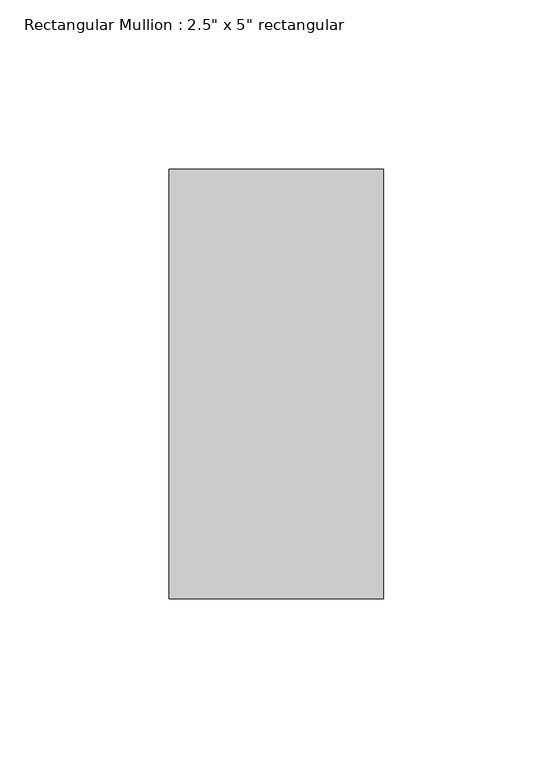
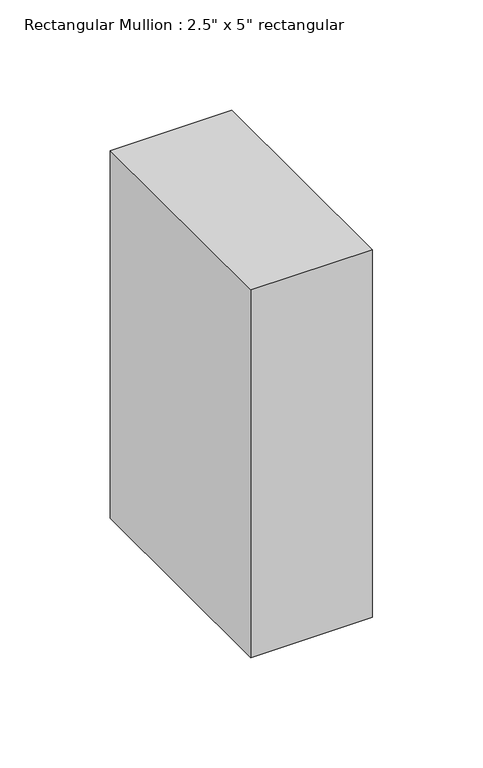
"""IFC4 building model written with IfcOpenShell, lengths in millimetres: member geometry."""

from ifc_helpers import new_model, si_unit, frame, origin, place, context, project, spatial, polyline, outline, extrude, source, transform, mapped, element, save


def member_a8054089(model_context):
    return source(origin(), model_context, "Body", "SweptSolid", [
        extrude(outline(polyline([(0.0, 63.5), (0.0, -63.5), (-63.5, -63.5), (-63.5, 63.5), (0.0, 63.5)])), frame((0.0, 0.0, -203.2), z_axis=(0.0, 0.0, 1.0), x_axis=(1.0, 0.0, 0.0)), (0.0, 0.0, 1.0), 203.2),
    ])


if __name__ == "__main__":
    model = new_model("IFC4")
    model_context = context("Model", 3, world=origin())
    ifc_project = project(units=[si_unit("LENGTHUNIT", "METRE", prefix="MILLI")], contexts=[model_context])
    site = spatial("IfcSite", under=ifc_project)
    building = spatial("IfcBuilding", under=site)
    placement = place(None, origin())
    member_shape = member_a8054089(model_context)
    element("IfcMember", 1, ObjectType="Rectangular Mullion : 2.5\" x 5\" rectangular", at=placement, inside=building, context=model_context, shape_type="MappedRepresentation", body=[
        mapped(member_shape, transform((0.0, 0.0, 0.0), x_axis=(1.0, 0.0, 0.0), y_axis=(0.0, 1.0, 0.0), z_axis=(0.0, 0.0, 1.0))),
    ])
    save(model, "model.ifc")

# Revit data of these elements
# Type "Rectangular Mullion : 2.5\" x 5\" rectangular"
#   built-in parameter 1007304 = 0.416667 (stored number, unit not read)
#   built-in parameter 1007301 = 0.104167 (stored number, unit not read)
#   built-in parameter 1007300 = 0.104167 (stored number, unit not read)
# Element 1 (IfcMember, "Rectangular Mullion : 2.5\" x 5\" rectangular")
#   Materials on its faces: "Door - Frame"
# Materials
#   "Door - Frame": colour RGB 118 70 51, transparency 0, Cost = 0
